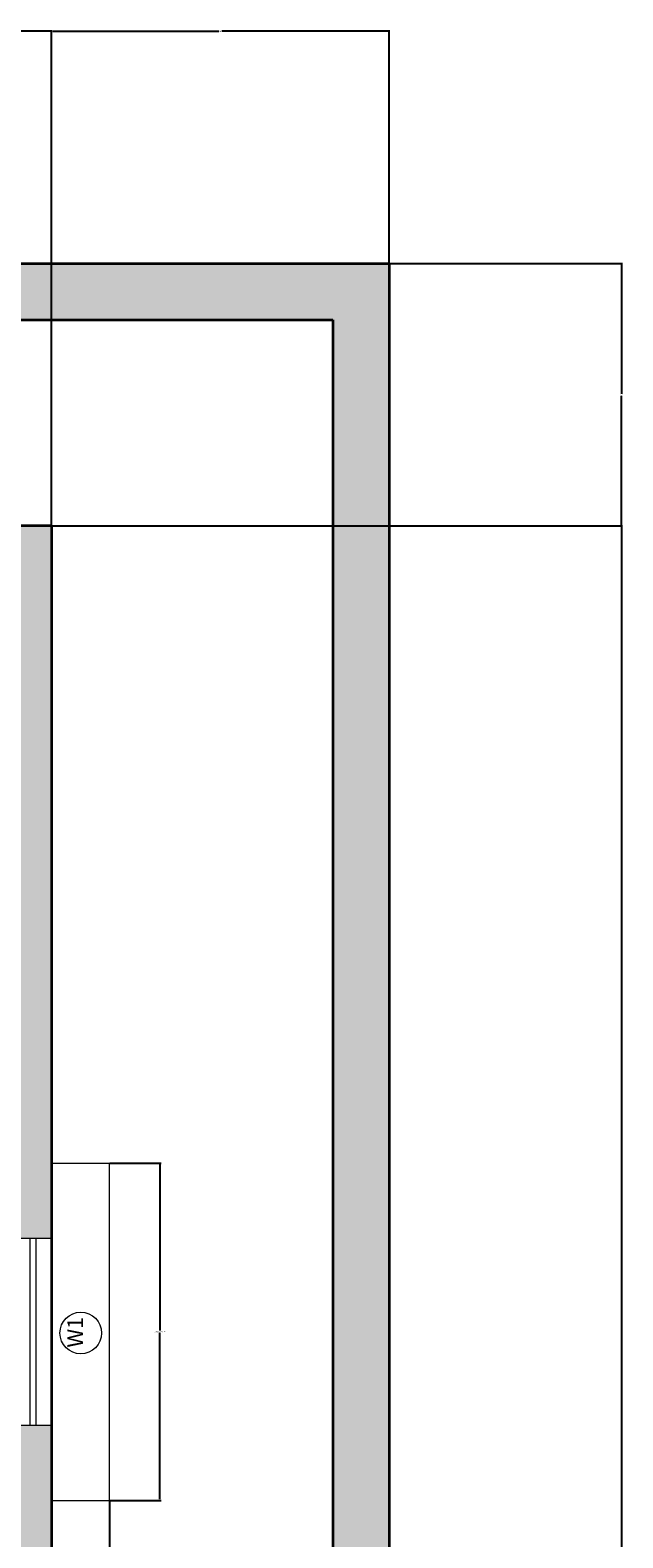
# Model space of a CAD drawing. Units: inches. Extents: x 2701 to 6846, y 811 to 2447.
# Tile 20 of 20: x 3089 to 3183, y 1300 to 1541. Entities that reach past the tile are written whole.
import ezdxf

# ---------------------------------------------------------------- set-up
doc = ezdxf.new("R2010")
doc.units = ezdxf.units.IN
for name, color, linetype, lineweight in [('A-ANNO-DIMS', 2, 'Continuous', 18), ('A-GLAZ', 4, 'Continuous', 18), ('A-WALL', 7, 'Continuous', 35), ('C-PROP', 7, 'Continuous', 35)]:
    doc.layers.add(name, color=color, linetype=linetype, lineweight=lineweight)
doc.layers.add('A-WALL-PATT', color=18, linetype='Continuous', lineweight=13, true_color=0x000000)
doc.layers.add('C-PROP-PATT', color=18, linetype='Continuous', lineweight=13, true_color=0x000000)
doc.styles.get("Standard").update_dxf_attribs({"font": 'arial.ttf'})
doc.dimstyles.get("Standard").update_dxf_attribs({"dimtxt": 0.18, "dimasz": 0.18, "dimexe": 0.18, "dimexo": 0.0625, "dimgap": 0.09, "dimtad": 0, "dimtih": 1, "dimtoh": 1, "dimdec": 4, "dimzin": 0, "dimdsep": 46, "dimtxsty": 'Standard', "dimcen": 0.09, "dimadec": 0, "dimazin": 0, "dimtfac": 1, "dimtdec": 4, "dimtofl": 0, "dimtmove": 0, "dimatfit": 3, "dimfxl": 1, "dimtolj": 1, "dimtzin": 0, "dimarcsym": 0})

# ---------------------------------------------------------------- blocks, each defined once
blk = doc.blocks.new('W1')
for p, q in [((3091.97, 1348.05), (3091.97, 1360.05)), ((3091.97, 1360.05), (3091.97, 1358.83)), ((3091.97, 1360.05), (3101.22, 1360.05)), ((3101.22, 1306.05), (3101.22, 1360.05)), ((3085.97, 1318.05), (3085.97, 1348.05)), ((3085.97, 1348.05), (3091.97, 1348.05)), ((3088.47, 1348.05), (3088.47, 1318.05)), ((3089.47, 1348.05), (3089.47, 1318.05)), ((3091.97, 1348.05), (3091.97, 1348.05)), ((3091.97, 1348.05), (3091.97, 1318.05)), ((3091.97, 1318.05), (3085.97, 1318.05)), ((3091.97, 1318.05), (3091.97, 1306.05)), ((3091.97, 1306.05), (3091.97, 1306.05)), ((3091.97, 1306.05), (3101.22, 1306.05))]:
    blk.add_line(p, q)
blk.add_circle((3096.65, 1332.84), 3.33)
at = {"insert": (3097.78, 1330.51), "char_height": 2.5, "attachment_point": 7, "rotation": 90}
blk.add_mtext('W1', dxfattribs=at)
blk = doc.blocks.new('*D33')
at = {"layer": 'A-ANNO-DIMS', "color": 0, "lineweight": -2, "transparency": 16777216}
for p, q in [((3101.28, 1360.05), (3109.5, 1360.05)), ((3109.32, 1359.87), (3109.32, 1333.23)), ((3109.32, 1306.23), (3109.32, 1332.87)), ((3101.28, 1306.05), (3109.5, 1306.05))]:
    blk.add_line(p, q, dxfattribs=at)
at = {"layer": 'A-ANNO-DIMS', "color": 0, "transparency": 16777216}
for points in [[(3109.29, 1359.87), (3109.35, 1359.87), (3109.32, 1360.05)], [(3109.29, 1306.23), (3109.35, 1306.23), (3109.32, 1306.05)]]:
    blk.add_solid(points, dxfattribs=at)
at = {"layer": 'Defpoints', "color": 0, "transparency": 16777216}
for p in [(3101.22, 1360.05), (3109.32, 1360.05), (3101.22, 1306.05)]:
    blk.add_point(p, dxfattribs=at)
at = {"layer": 'A-ANNO-DIMS', "color": 0, "transparency": 16777216, "insert": (3109.32, 1333.05), "char_height": 0.18, "attachment_point": 5}
blk.add_mtext('\\A1;WINDOW W1 54', dxfattribs=at)
blk = doc.blocks.new('*D34')
at = {"layer": 'A-ANNO-DIMS', "color": 0, "lineweight": -2, "transparency": 16777216}
for p, q in [((3085.97, 1305.99), (3085.97, 1297.77)), ((3101.22, 1305.99), (3101.22, 1297.77)), ((3086.15, 1297.95), (3093.38, 1297.95)), ((3101.04, 1297.95), (3093.81, 1297.95))]:
    blk.add_line(p, q, dxfattribs=at)
at = {"layer": 'A-ANNO-DIMS', "color": 0, "transparency": 16777216}
for points in [[(3086.15, 1297.98), (3086.15, 1297.92), (3085.97, 1297.95)], [(3101.04, 1297.98), (3101.04, 1297.92), (3101.22, 1297.95)]]:
    blk.add_solid(points, dxfattribs=at)
at = {"layer": 'Defpoints', "color": 0, "transparency": 16777216}
for p in [(3085.97, 1306.05), (3101.22, 1306.05), (3101.22, 1297.95)]:
    blk.add_point(p, dxfattribs=at)
at = {"layer": 'A-ANNO-DIMS', "color": 0, "transparency": 16777216, "insert": (3093.59, 1297.95), "char_height": 0.18, "attachment_point": 5}
blk.add_mtext('\\A1;15', dxfattribs=at)
blk = doc.blocks.new('*D67')
at = {"layer": 'A-ANNO-DIMS', "color": 0, "lineweight": -2, "transparency": 16777216}
for p, q in [((2779.97, 1462.11), (2779.97, 1541.43)), ((2780.15, 1541.25), (2935.68, 1541.25)), ((3091.79, 1541.25), (2936.26, 1541.25)), ((3091.97, 1462.11), (3091.97, 1541.43))]:
    blk.add_line(p, q, dxfattribs=at)
at = {"layer": 'A-ANNO-DIMS', "color": 0, "transparency": 16777216}
for points in [[(2780.15, 1541.28), (2780.15, 1541.22), (2779.97, 1541.25)], [(3091.79, 1541.28), (3091.79, 1541.22), (3091.97, 1541.25)]]:
    blk.add_solid(points, dxfattribs=at)
at = {"layer": 'Defpoints', "color": 0, "transparency": 16777216}
for p in [(3091.97, 1541.25), (2779.97, 1462.05), (3091.97, 1462.05)]:
    blk.add_point(p, dxfattribs=at)
at = {"layer": 'A-ANNO-DIMS', "color": 0, "transparency": 16777216, "insert": (2935.97, 1541.25), "char_height": 0.18, "attachment_point": 5}
blk.add_mtext('\\A1;312', dxfattribs=at)
blk = doc.blocks.new('*D68')
at = {"layer": 'A-ANNO-DIMS', "color": 0, "lineweight": -2, "transparency": 16777216}
for p, q in [((3092.03, 1462.05), (3183.35, 1462.05)), ((3183.17, 1461.87), (3183.17, 1246.23)), ((3183.17, 1030.23), (3183.17, 1245.87)), ((3092.03, 1030.05), (3183.35, 1030.05))]:
    blk.add_line(p, q, dxfattribs=at)
at = {"layer": 'A-ANNO-DIMS', "color": 0, "transparency": 16777216}
for points in [[(3183.14, 1461.87), (3183.2, 1461.87), (3183.17, 1462.05)], [(3183.14, 1030.23), (3183.2, 1030.23), (3183.17, 1030.05)]]:
    blk.add_solid(points, dxfattribs=at)
at = {"layer": 'Defpoints', "color": 0, "transparency": 16777216}
for p in [(3091.97, 1462.05), (3183.17, 1462.05), (3091.97, 1030.05)]:
    blk.add_point(p, dxfattribs=at)
at = {"layer": 'A-ANNO-DIMS', "color": 0, "transparency": 16777216, "insert": (3183.17, 1246.05), "char_height": 0.18, "attachment_point": 5}
blk.add_mtext('\\A1;432', dxfattribs=at)
blk = doc.blocks.new('*D71')
at = {"layer": 'A-ANNO-DIMS', "color": 0, "lineweight": -2, "transparency": 16777216}
for p, q in [((3146.03, 1504.05), (3183.35, 1504.05)), ((3183.17, 1503.87), (3183.17, 1483.23)), ((3183.17, 1462.23), (3183.17, 1482.87)), ((3092.03, 1462.05), (3183.35, 1462.05))]:
    blk.add_line(p, q, dxfattribs=at)
at = {"layer": 'A-ANNO-DIMS', "color": 0, "transparency": 16777216}
for points in [[(3183.14, 1503.87), (3183.2, 1503.87), (3183.17, 1504.05)], [(3183.14, 1462.23), (3183.2, 1462.23), (3183.17, 1462.05)]]:
    blk.add_solid(points, dxfattribs=at)
at = {"layer": 'Defpoints', "color": 0, "transparency": 16777216}
for p in [(3145.97, 1504.05), (3183.17, 1504.05), (3091.97, 1462.05)]:
    blk.add_point(p, dxfattribs=at)
at = {"layer": 'A-ANNO-DIMS', "color": 0, "transparency": 16777216, "insert": (3183.17, 1483.05), "char_height": 0.18, "attachment_point": 5}
blk.add_mtext('\\A1;42', dxfattribs=at)
blk = doc.blocks.new('*D72')
at = {"layer": 'A-ANNO-DIMS', "color": 0, "lineweight": -2, "transparency": 16777216}
for p, q in [((3091.97, 1462.11), (3091.97, 1541.43)), ((3092.15, 1541.25), (3118.75, 1541.25)), ((3145.79, 1541.25), (3119.19, 1541.25)), ((3145.97, 1504.11), (3145.97, 1541.43))]:
    blk.add_line(p, q, dxfattribs=at)
at = {"layer": 'A-ANNO-DIMS', "color": 0, "transparency": 16777216}
for points in [[(3092.15, 1541.28), (3092.15, 1541.22), (3091.97, 1541.25)], [(3145.79, 1541.28), (3145.79, 1541.22), (3145.97, 1541.25)]]:
    blk.add_solid(points, dxfattribs=at)
at = {"layer": 'Defpoints', "color": 0, "transparency": 16777216}
for p in [(3145.97, 1541.25), (3145.97, 1504.05), (3091.97, 1462.05)]:
    blk.add_point(p, dxfattribs=at)
at = {"layer": 'A-ANNO-DIMS', "color": 0, "transparency": 16777216, "insert": (3118.97, 1541.25), "char_height": 0.18, "attachment_point": 5}
blk.add_mtext('\\A1;54', dxfattribs=at)

msp = doc.modelspace()

# ---------------------------------------------------------------- hatches: boundary and pattern name
at = {"layer": 'A-WALL-PATT'}
h = msp.add_hatch(color=256, dxfattribs=at)
h.dxf.hatch_style = 1
h.paths.add_polyline_path([(3085.97, 1456.05), (3085.97, 1348.05), (3091.97, 1348.05), (3091.97, 1360.05), (3091.97, 1462.05), (2960.09, 1462.05), (2960.09, 1456.05), (2971.97, 1456.05), (2971.97, 1372.05), (2923.97, 1372.05), (2923.97, 1378.05), (2917.97, 1378.05), (2917.97, 1351.05), (2923.97, 1351.05), (2923.97, 1366.05), (2971.97, 1366.05), (2971.97, 1351.05), (2976.77, 1351.05), (2977.97, 1351.05), (2977.97, 1456.05)])
h.paths.add_polyline_path([(2779.97, 1462.05), (2779.97, 1342.05), (2785.97, 1342.05), (2785.97, 1456.05), (2917.97, 1456.05), (2917.97, 1408.05), (2922.33, 1408.05), (2923.97, 1408.05), (2923.97, 1456.05), (2937.09, 1456.05), (2937.09, 1462.05)])
h.paths.add_polyline_path([(2779.97, 1306.05), (2779.97, 1294.24), (2785.97, 1294.24), (2785.97, 1306.05), (2851.37, 1306.05, -0.025815), (2852.62, 1306.11, -0.025815), (2853.87, 1306.05), (2863.97, 1306.05), (2863.97, 1258.05), (2857.97, 1258.05), (2857.97, 1252.05), (2878.97, 1252.05), (2878.97, 1258.05), (2869.97, 1258.05), (2869.97, 1306.05), (2923.97, 1306.05), (2923.97, 1318.05), (2919.17, 1318.05), (2917.97, 1318.05), (2917.97, 1312.05), (2785.97, 1312.05), (2785.97, 1318.05), (2779.97, 1318.05)])
h.paths.add_polyline_path([(2785.97, 1252.05), (2827.97, 1252.05), (2827.97, 1256.41), (2827.97, 1258.05), (2785.97, 1258.05), (2785.97, 1271.24), (2779.97, 1271.24), (2779.97, 1174.05), (2785.97, 1174.05)])
h.paths.add_polyline_path([(2779.97, 1030.05), (2869.97, 1030.05), (2869.97, 1036.05), (2785.97, 1036.05), (2785.97, 1126.05), (2917.97, 1126.05), (2917.97, 1120.05), (2923.97, 1120.05), (2923.97, 1258.05), (2911.97, 1258.05), (2911.97, 1253.25), (2911.97, 1252.05), (2917.97, 1252.05), (2917.97, 1132.05), (2785.97, 1132.05), (2785.97, 1144.05), (2779.97, 1144.05)])
h.paths.add_polyline_path([(2935.97, 1030.05), (2935.97, 1033.05), (2935.97, 1036.05), (2923.97, 1036.05), (2923.97, 1087.05), (2919.17, 1087.05), (2917.97, 1087.05), (2917.97, 1036.05), (2893.97, 1036.05), (2893.97, 1030.05)])
h.paths.add_polyline_path([(2971.97, 1036.05), (2971.97, 1030.05), (3091.97, 1030.05), (3091.97, 1060.05), (3085.97, 1060.05), (3085.97, 1036.05)])
h.paths.add_polyline_path([(3085.97, 1084.05), (3091.97, 1084.05), (3091.97, 1096.05), (3091.97, 1268.89), (3085.97, 1268.89), (3085.97, 1258.05), (3001.97, 1258.05), (3001.97, 1270.05), (2995.97, 1270.05), (2995.97, 1252.05), (3085.97, 1252.05)])
h.paths.add_polyline_path([(3085.97, 1306.05), (3085.97, 1291.89), (3091.97, 1291.89), (3091.97, 1318.05), (3085.97, 1318.05), (3085.97, 1312.05), (2977.97, 1312.05), (2977.97, 1318.05), (2971.97, 1318.05), (2971.97, 1306.05), (2995.97, 1306.05), (2995.97, 1300.05), (3000.33, 1300.05), (3001.97, 1300.05), (3001.97, 1306.05)])
at = {"layer": 'C-PROP-PATT'}
h = msp.add_hatch(color=256, dxfattribs=at)
h.dxf.hatch_style = 1
h.paths.add_polyline_path([(3145.97, 1504.05), (2737.97, 1504.05), (2737.97, 967.05), (2746.97, 967.05), (2746.97, 1495.05), (3136.97, 1495.05), (3136.97, 865.05), (3130.97, 865.05), (3130.97, 856.05), (3145.97, 856.05)])
h.paths.add_polyline_path([(3070.97, 865.05), (2746.97, 865.05), (2746.97, 871.05), (2737.97, 871.05), (2737.97, 856.05), (3070.97, 856.05)], flags=17)

# ---------------------------------------------------------------- linework, layer by layer
at = {"layer": 'A-WALL'}
for q in [(2779.97, 1462.05), (3091.97, 1030.05)]:
    msp.add_line((3091.97, 1462.05), q, dxfattribs=at)
at = {"layer": 'C-PROP'}
for p, q in [((2737.97, 1504.05), (3145.97, 1504.05)), ((3145.97, 1504.05), (3145.97, 856.05)), ((2746.97, 1495.05), (3136.97, 1495.05)), ((3136.97, 1495.05), (3136.97, 865.05))]:
    msp.add_line(p, q, dxfattribs=at)

# ---------------------------------------------------------------- block references
at = {"layer": 'A-GLAZ'}
msp.add_blockref('W1', (0, 0), dxfattribs=at)

# ---------------------------------------------------------------- dimensions: what is measured, and where the dimension line sits
at = {"layer": 'A-ANNO-DIMS'}
for base, p1, p2, picture, middle in [((3091.97, 1541.25), (2779.97, 1462.05), (3091.97, 1462.05), '*D67', (2935.97, 1541.25)), ((3145.97, 1541.25), (3091.97, 1462.05), (3145.97, 1504.05), '*D72', (3118.97, 1541.25)), ((3101.22, 1297.95), (3085.97, 1306.05), (3101.22, 1306.05), '*D34', (3093.59, 1297.95))]:
    dim = msp.add_linear_dim(base=base, p1=p1, p2=p2, dimstyle='Standard', override={"dimdec": 0, "dimlfac": 1, "dimrnd": 0, "dimzin": 0, "dimdsep": 46, "dimlunit": 2}, dxfattribs=at)
    dim.commit()
    dim.dimension.update_dxf_attribs({"geometry": picture, "text_midpoint": middle})
for base, p1, p2, picture, middle in [((3183.17, 1504.05), (3091.97, 1462.05), (3145.97, 1504.05), '*D71', (3183.17, 1483.05)), ((3183.17, 1462.05), (3091.97, 1030.05), (3091.97, 1462.05), '*D68', (3183.17, 1246.05))]:
    dim = msp.add_linear_dim(base=base, p1=p1, p2=p2, angle=90, dimstyle='Standard', override={"dimdec": 0, "dimlfac": 1, "dimrnd": 0, "dimzin": 0, "dimdsep": 46, "dimlunit": 2}, dxfattribs=at)
    dim.commit()
    dim.dimension.update_dxf_attribs({"geometry": picture, "text_midpoint": middle})
dim = msp.add_linear_dim(base=(3109.32, 1360.05), p1=(3101.22, 1306.05), p2=(3101.22, 1360.05), angle=90, text='WINDOW W1 <>', dimstyle='Standard', override={"dimdec": 0, "dimlfac": 1, "dimrnd": 0, "dimzin": 0, "dimdsep": 46, "dimlunit": 2}, dxfattribs=at)
dim.commit()
dim.dimension.update_dxf_attribs({"geometry": '*D33', "text_midpoint": (3109.32, 1333.05)})

doc.saveas('drawing.dxf')
